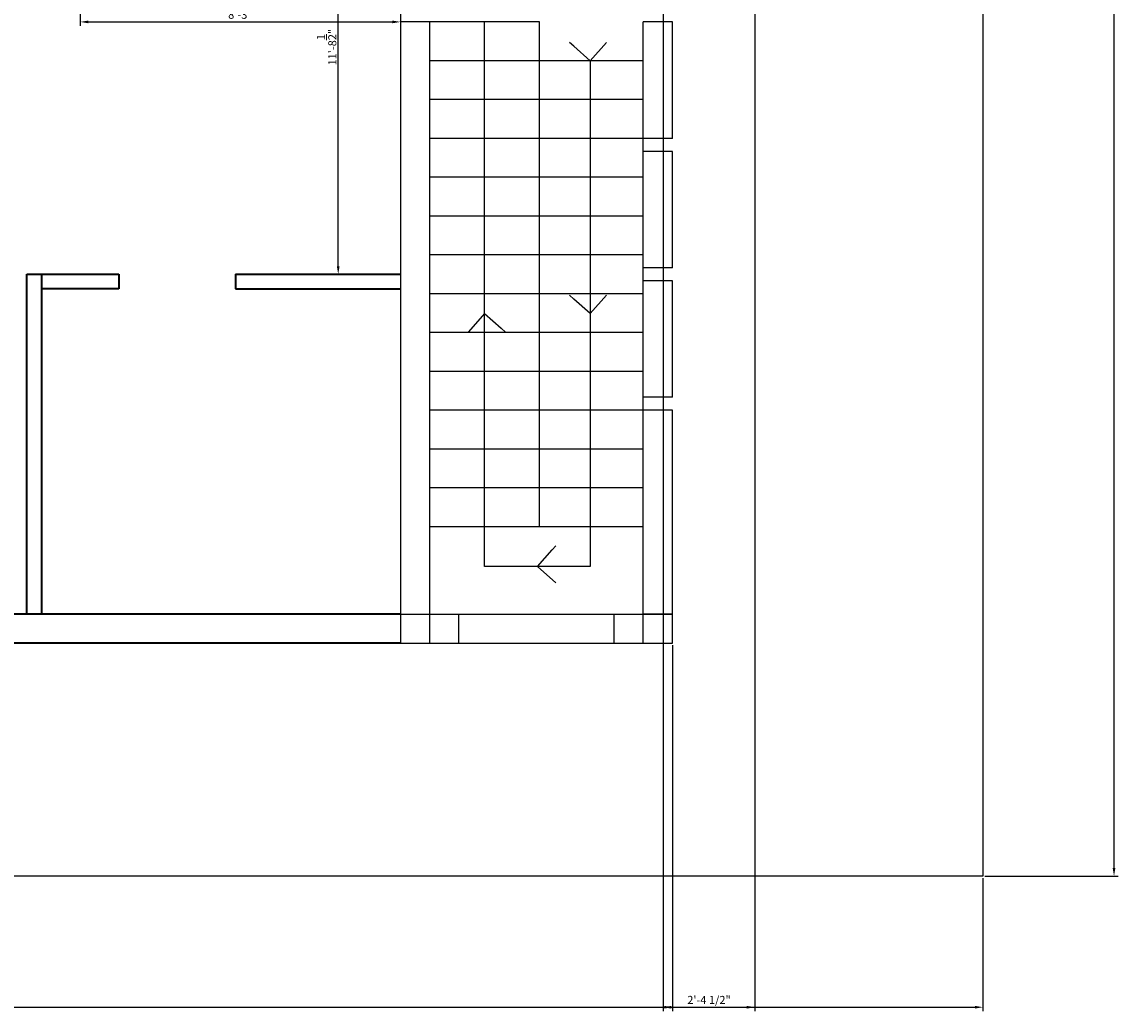
# Model space of a CAD drawing. Units: inches. Extents: x 250205121 to 250208111, y 89832590 to 89833271.
# Tile 8 of 14: x 250206724 to 250207062, y 89832600 to 89832906. Entities that reach past the tile are written whole.
import ezdxf

# ---------------------------------------------------------------- set-up
doc = ezdxf.new("R2010")
doc.units = ezdxf.units.IN
for name, color, linetype, lineweight in [('A-FLOR-STRS', 7, 'Continuous', 25), ('A-WALL', 7, 'Continuous', 35), ('C-PROP', 8, 'Continuous', 25), ('dimensions', 2, 'Continuous', 18)]:
    doc.layers.add(name, color=color, linetype=linetype, lineweight=lineweight)
doc.styles.get("Standard").update_dxf_attribs({"font": 'arial.ttf'})
doc.dimstyles.new('ISO-25', dxfattribs={"dimtxt": 2.5, "dimasz": 2.5, "dimexe": 1.25, "dimexo": 0.625, "dimtad": 1, "dimlunit": 4, "dimtxsty": 'Standard', "dimcen": 2.5, "dimadec": 0, "dimazin": 0, "dimtfac": 1, "dimtmove": 0, "dimatfit": 3, "dimfxl": 1, "dimarcsym": 0})

# ---------------------------------------------------------------- blocks, each defined once
blk = doc.blocks.new('*D17')
at = {"layer": 'Defpoints', "color": 0, "transparency": 16777216}
for p in [(250206741.69, 89832968.74), (250206840.69, 89832968.74), (250206840.69, 89832906.33)]:
    blk.add_point(p, dxfattribs=at)
at = {"layer": 'dimensions', "color": 0, "lineweight": -2, "transparency": 16777216}
for p, q in [((250206741.69, 89832968.12), (250206741.69, 89832905.08)), ((250206840.69, 89832968.12), (250206840.69, 89832905.08)), ((250206744.19, 89832906.33), (250206838.19, 89832906.33))]:
    blk.add_line(p, q, dxfattribs=at)
at = {"layer": 'dimensions', "color": 0, "transparency": 16777216}
for points in [[(250206744.19, 89832906.74), (250206744.19, 89832905.91), (250206741.69, 89832906.33)], [(250206838.19, 89832906.74), (250206838.19, 89832905.91), (250206840.69, 89832906.33)]]:
    blk.add_solid(points, dxfattribs=at)
at = {"layer": 'dimensions', "color": 0, "transparency": 16777216, "insert": (250206791.19, 89832908.23), "char_height": 2.5, "attachment_point": 5}
blk.add_mtext('8\'-3"', dxfattribs=at)
blk = doc.blocks.new('*D18')
at = {"layer": 'Defpoints', "color": 0, "transparency": 16777216}
for p in [(250206821.44, 89832968.74), (250206823.27, 89832968.74), (250206823.27, 89832828.33)]:
    blk.add_point(p, dxfattribs=at)
at = {"layer": 'dimensions', "color": 0, "lineweight": -2, "transparency": 16777216}
for p, q in [((250206822.65, 89832968.74), (250206820.19, 89832968.74)), ((250206821.44, 89832830.83), (250206821.44, 89832966.24)), ((250206822.65, 89832828.33), (250206820.19, 89832828.33))]:
    blk.add_line(p, q, dxfattribs=at)
at = {"layer": 'dimensions', "color": 0, "transparency": 16777216}
for points in [[(250206821.02, 89832966.24), (250206821.85, 89832966.24), (250206821.44, 89832968.74)], [(250206821.02, 89832830.83), (250206821.85, 89832830.83), (250206821.44, 89832828.33)]]:
    blk.add_solid(points, dxfattribs=at)
at = {"layer": 'dimensions', "color": 0, "transparency": 16777216, "insert": (250206817.86, 89832898.53), "char_height": 2.5, "attachment_point": 5, "rotation": 90}
blk.add_mtext('11\'-8{\\H1x;\\S1/2;}"', dxfattribs=at)
blk = doc.blocks.new('STAIR-RETURN')
for p, q in [((9, 192), (0, 192)), ((0, 192), (0, 0)), ((43, 192), (9, 192)), ((9, 192), (9, 0)), ((26, 23.7), (26, 192)), ((43, 36), (43, 192)), ((84, 192), (75, 192)), ((75, 0), (75, 192)), ((84, 156), (84, 192)), ((53.53, 184.53), (52.21, 185.69)), ((58.64, 180), (53.53, 184.53)), ((58.64, 180), (63.65, 185.66)), ((75, 180), (9, 180)), ((58.64, 180), (58.64, 23.7)), ((75, 168), (9, 168)), ((75, 156), (9, 156)), ((84, 156), (75, 156)), ((84, 152), (75, 152)), ((84, 116), (84, 152)), ((75, 144), (9, 144)), ((75, 132), (9, 132)), ((75, 120), (9, 120)), ((84, 116), (75, 116)), ((84, 112), (75, 112)), ((84, 76), (84, 112)), ((75, 108), (9, 108)), ((53.53, 106.37), (52.21, 107.54)), ((58.64, 101.85), (53.53, 106.37)), ((58.64, 101.85), (63.65, 107.51)), ((26, 101.85), (20.99, 96.18)), ((26, 101.85), (31.11, 97.32)), ((75, 96), (9, 96)), ((31.11, 97.32), (32.43, 96.16)), ((75, 84), (9, 84)), ((84, 76), (75, 76)), ((75, 72), (9, 72)), ((84, 72), (75, 72)), ((84, 0), (84, 72)), ((75, 60), (9, 60)), ((75, 48), (9, 48)), ((75, 36), (9, 36)), ((42.32, 23.7), (46.85, 28.81)), ((46.85, 28.81), (48.01, 30.12)), ((58.64, 23.7), (26, 23.7)), ((42.32, 23.7), (47.98, 18.68)), ((0, 9), (84, 9)), ((18, 0), (18, 9)), ((66, 0), (66, 9)), ((84, 9), (75, 9)), ((0, 0), (84, 0))]:
    blk.add_line(p, q)
blk = doc.blocks.new('STAIR-CENTRAL')
for p, q in [((0, 105), (30, 105)), ((30, 105), (30, 0)), ((30, 105), (151.5, 105)), ((42.15, 105), (42.15, 0)), ((54.3, 105), (54.3, 0)), ((66.45, 105), (66.45, 0)), ((78.6, 105), (78.6, 0)), ((90.75, 105), (90.75, 0)), ((102.9, 105), (102.9, 0)), ((115.05, 105), (115.05, 0)), ((127.2, 105), (127.2, 0)), ((139.35, 105), (139.35, 0)), ((151.5, 105), (151.5, 0)), ((151.5, 105), (151.5, 0)), ((151.5, 52.5), (30, 52.5)), ((0, 0), (6, 0)), ((6, 0), (30, 0)), ((30, 0), (151.5, 0)), ((151.5, 0), (175.5, 0)), ((175.5, 0), (181.5, 0))]:
    blk.add_line(p, q)
blk = doc.blocks.new('*D54')
at = {"layer": 'Defpoints', "color": 0, "transparency": 16777216}
for p in [(250206218.19, 89832642.33), (250207020.69, 89832642.33), (250207020.69, 89832601.83)]:
    blk.add_point(p, dxfattribs=at)
at = {"layer": 'dimensions', "color": 0, "lineweight": -2, "transparency": 16777216}
for p, q in [((250206218.19, 89832641.7), (250206218.19, 89832600.58)), ((250207020.69, 89832641.7), (250207020.69, 89832600.58)), ((250206220.69, 89832601.83), (250207018.19, 89832601.83))]:
    blk.add_line(p, q, dxfattribs=at)
at = {"layer": 'dimensions', "color": 0, "transparency": 16777216}
for points in [[(250206220.69, 89832602.24), (250206220.69, 89832601.41), (250206218.19, 89832601.83)], [(250207018.19, 89832602.24), (250207018.19, 89832601.41), (250207020.69, 89832601.83)]]:
    blk.add_solid(points, dxfattribs=at)
at = {"layer": 'dimensions', "color": 0, "transparency": 16777216, "insert": (250206619.44, 89832603.75), "char_height": 2.5, "attachment_point": 5}
blk.add_mtext('66\'-10 1/2"', dxfattribs=at)
blk = doc.blocks.new('*D55')
at = {"layer": 'Defpoints', "color": 0, "transparency": 16777216}
for p in [(250207020.69, 89833215.33), (250207061.19, 89833215.33), (250207020.69, 89832642.33)]:
    blk.add_point(p, dxfattribs=at)
at = {"layer": 'dimensions', "color": 0, "lineweight": -2, "transparency": 16777216}
for p, q in [((250207021.31, 89833215.33), (250207062.44, 89833215.33)), ((250207061.19, 89832644.83), (250207061.19, 89833212.83)), ((250207021.31, 89832642.33), (250207062.44, 89832642.33))]:
    blk.add_line(p, q, dxfattribs=at)
at = {"layer": 'dimensions', "color": 0, "transparency": 16777216}
for points in [[(250207060.77, 89833212.83), (250207061.6, 89833212.83), (250207061.19, 89833215.33)], [(250207060.77, 89832644.83), (250207061.6, 89832644.83), (250207061.19, 89832642.33)]]:
    blk.add_solid(points, dxfattribs=at)
at = {"layer": 'dimensions', "color": 0, "transparency": 16777216, "insert": (250207059.29, 89832928.83), "char_height": 2.5, "attachment_point": 5, "rotation": 90}
blk.add_mtext('47\'-9"', dxfattribs=at)
blk = doc.blocks.new('*D61')
at = {"layer": 'Defpoints', "color": 0, "transparency": 16777216}
for p in [(250206290.19, 89832714.33), (250206924.69, 89832714.33), (250206924.69, 89832601.83)]:
    blk.add_point(p, dxfattribs=at)
at = {"layer": 'dimensions', "color": 0, "lineweight": -2, "transparency": 16777216}
for p, q in [((250206290.19, 89832713.7), (250206290.19, 89832600.58)), ((250206924.69, 89832713.7), (250206924.69, 89832600.58)), ((250206292.69, 89832601.83), (250206922.19, 89832601.83))]:
    blk.add_line(p, q, dxfattribs=at)
at = {"layer": 'dimensions', "color": 0, "transparency": 16777216}
for points in [[(250206292.69, 89832602.24), (250206292.69, 89832601.41), (250206290.19, 89832601.83)], [(250206922.19, 89832602.24), (250206922.19, 89832601.41), (250206924.69, 89832601.83)]]:
    blk.add_solid(points, dxfattribs=at)
at = {"layer": 'dimensions', "color": 0, "transparency": 16777216, "insert": (250206607.44, 89832603.75), "char_height": 2.5, "attachment_point": 5}
blk.add_mtext('52\'-10 1/2"', dxfattribs=at)
blk = doc.blocks.new('*D62')
at = {"layer": 'Defpoints', "color": 0, "transparency": 16777216}
for p in [(250206921.85, 89833047.33), (250206950.19, 89833047.33), (250206950.19, 89832601.83)]:
    blk.add_point(p, dxfattribs=at)
at = {"layer": 'dimensions', "color": 0, "lineweight": -2, "transparency": 16777216}
for p, q in [((250206921.85, 89833046.7), (250206921.85, 89832600.58)), ((250206950.19, 89833046.7), (250206950.19, 89832600.58)), ((250206924.35, 89832601.83), (250206947.69, 89832601.83))]:
    blk.add_line(p, q, dxfattribs=at)
at = {"layer": 'dimensions', "color": 0, "transparency": 16777216}
for points in [[(250206924.35, 89832602.24), (250206924.35, 89832601.41), (250206921.85, 89832601.83)], [(250206947.69, 89832602.24), (250206947.69, 89832601.41), (250206950.19, 89832601.83)]]:
    blk.add_solid(points, dxfattribs=at)
at = {"layer": 'dimensions', "color": 0, "transparency": 16777216, "insert": (250206936.02, 89832603.75), "char_height": 2.5, "attachment_point": 5}
blk.add_mtext('2\'-4 1/2"', dxfattribs=at)

msp = doc.modelspace()

# ---------------------------------------------------------------- linework, layer by layer
at = {"layer": 'A-WALL'}
for p, q in [((250206725.187, 89832723.328), (250206725.187, 89832828.328)), ((250206725.187, 89832828.328), (250206729.687, 89832828.328)), ((250206729.687, 89832828.328), (250206729.687, 89832723.328)), ((250206729.687, 89832828.328), (250206753.687, 89832828.328)), ((250206753.687, 89832828.328), (250206753.687, 89832823.828)), ((250206789.687, 89832828.328), (250206789.687, 89832823.828)), ((250206789.687, 89832828.328), (250206840.687, 89832828.328)), ((250206753.687, 89832823.828), (250206729.687, 89832823.828)), ((250206789.687, 89832823.828), (250206840.687, 89832823.828)), ((250206840.687, 89832723.328), (250206299.187, 89832723.328)), ((250206840.687, 89832714.328), (250206307.687, 89832714.328))]:
    msp.add_line(p, q, dxfattribs=at)
at = {"layer": 'C-PROP'}
for p, q in [((250207020.687, 89833179.328), (250207020.687, 89832642.328)), ((250207020.687, 89832642.328), (250206543.687, 89832642.328))]:
    msp.add_line(p, q, dxfattribs=at)

# ---------------------------------------------------------------- block references
at = {"layer": 'A-FLOR-STRS'}
for name, p in [('STAIR-RETURN', (250206840.687, 89832714.328)), ('STAIR-CENTRAL', (250206543.687, 89832723.328))]:
    msp.add_blockref(name, p, dxfattribs=at)

# ---------------------------------------------------------------- dimensions: what is measured, and where the dimension line sits
at = {"layer": 'dimensions'}
for base, p1, p2, override, picture, middle in [((250207061.187, 89833215.328), (250207020.687, 89832642.328), (250207020.687, 89833215.328), {"dimdec": 1, "dimlfac": 1, "dimrnd": 0, "dimzin": 1, "dimdsep": 46, "dimlunit": 4, "dimfrac": 2}, '*D55', (250207059.286, 89832928.828)), ((250206821.437, 89832968.74), (250206823.271, 89832828.328), (250206823.271, 89832968.74), {"dimclrd": 0, "dimclre": 0, "dimclrt": 0}, '*D18', (250206817.864, 89832898.534))]:
    dim = msp.add_linear_dim(base=base, p1=p1, p2=p2, angle=90, dimstyle='ISO-25', override=override, dxfattribs=at)
    dim.commit()
    dim.dimension.update_dxf_attribs({"geometry": picture, "text_midpoint": middle})
for base, p1, p2, override, picture, middle in [((250206950.187, 89832601.828), (250206921.847, 89833047.328), (250206950.187, 89833047.328), {"dimdec": 1, "dimlfac": 1, "dimrnd": 0, "dimzin": 1, "dimdsep": 46, "dimlunit": 4, "dimfrac": 2}, '*D62', (250206936.017, 89832603.746)), ((250206840.687, 89832906.328), (250206741.687, 89832968.74), (250206840.687, 89832968.74), {"dimclrd": 0, "dimclre": 0, "dimclrt": 0}, '*D17', (250206791.187, 89832908.23)), ((250206924.687, 89832601.828), (250206290.187, 89832714.328), (250206924.687, 89832714.328), {"dimdec": 1, "dimlfac": 1, "dimrnd": 0, "dimzin": 1, "dimdsep": 46, "dimlunit": 4, "dimfrac": 2}, '*D61', (250206607.437, 89832603.746)), ((250207020.687, 89832601.828), (250206218.187, 89832642.328), (250207020.687, 89832642.328), {"dimdec": 1, "dimlfac": 1, "dimrnd": 0, "dimzin": 1, "dimdsep": 46, "dimlunit": 4, "dimfrac": 2}, '*D54', (250206619.437, 89832603.746))]:
    dim = msp.add_linear_dim(base=base, p1=p1, p2=p2, dimstyle='ISO-25', override=override, dxfattribs=at)
    dim.commit()
    dim.dimension.update_dxf_attribs({"geometry": picture, "text_midpoint": middle})

doc.saveas('drawing.dxf')
